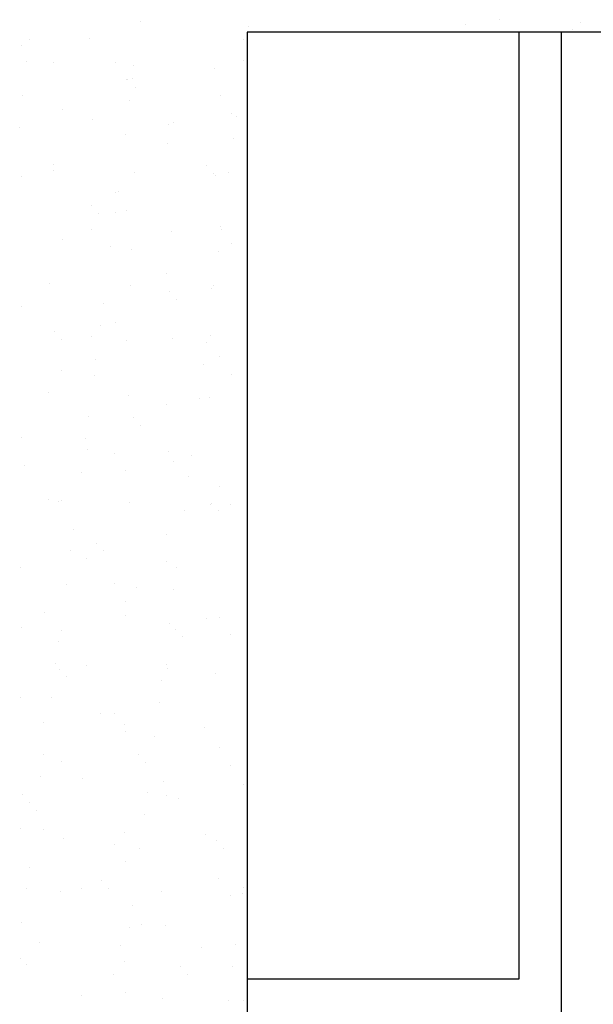
# Model space of a CAD drawing. Units: millimetres. Extents: x -857 to 54106, y -13666 to 13947.
# Tile 36 of 41: x 31477 to 32096, y 9453 to 10516. Entities that reach past the tile are written whole.
import ezdxf

# ---------------------------------------------------------------- set-up
doc = ezdxf.new("R2010")
doc.units = ezdxf.units.MM
for name, color, linetype in [('A-FRN', 11, 'Continuous'), ('A-HT', 15, 'Continuous'), ('L-HT', 1, 'Continuous')]:
    doc.layers.add(name, color=color, linetype=linetype)
doc.layers.add('A-FURN', color=21, linetype='Continuous', lineweight=18)

# ---------------------------------------------------------------- blocks, each defined once
blk = doc.blocks.new('*X18')
at = {"color": 0}
for p, q in [((1.2165, 2.3691), (1.2165, 2.3691)), ((1.2758, 2.3687), (1.2758, 2.3687)), ((1.3141, 2.3717), (1.3141, 2.3717)), ((1.3722, 2.3694), (1.3722, 2.3694)), ((1.5279, 2.3697), (1.5279, 2.3697)), ((1.6837, 2.37), (1.6837, 2.37)), ((1.7172, 2.3656), (1.7172, 2.3656)), ((1.8394, 2.3703), (1.8394, 2.3703)), ((1.911, 2.3696), (1.911, 2.3696)), ((1.9951, 2.3706), (1.9951, 2.3706)), ((2.1111, 2.3679), (2.1111, 2.3679)), ((2.1508, 2.3708), (2.1508, 2.3708)), ((2.264, 2.3694), (2.264, 2.3694)), ((2.3065, 2.3711), (2.3065, 2.3711)), ((1.2091, 2.36), (1.2091, 2.36)), ((1.2351, 2.3634), (1.2351, 2.3634)), ((2.1203, 2.3595), (2.1203, 2.3595)), ((2.1973, 2.3606), (2.1973, 2.3606)), ((2.2234, 2.364), (2.2234, 2.364)), ((2.3141, 2.3635), (2.3141, 2.3635)), ((1.8936, 2.3418), (1.8936, 2.3418)), ((2.0244, 2.3435), (2.0244, 2.3435)), ((2.0627, 2.3429), (2.0627, 2.3429)), ((2.0888, 2.3463), (2.0888, 2.3463)), ((2.1294, 2.3517), (2.1294, 2.3517)), ((2.1523, 2.3429), (2.1523, 2.3429)), ((2.2874, 2.3477), (2.2874, 2.3477)), ((1.2368, 2.3316), (1.2368, 2.3316)), ((1.3576, 2.3319), (1.3576, 2.3319)), ((1.3647, 2.331), (1.3647, 2.331)), ((1.4997, 2.3359), (1.4997, 2.3359)), ((1.5577, 2.3302), (1.5577, 2.3302)), ((1.6306, 2.3375), (1.6306, 2.3375)), ((1.7585, 2.3369), (1.7585, 2.3369)), ((1.9948, 2.3339), (1.9948, 2.3339)), ((1.2924, 2.3208), (1.2924, 2.3208)), ((1.4481, 2.3211), (1.4481, 2.3211)), ((1.5669, 2.3217), (1.5669, 2.3217)), ((1.6038, 2.3214), (1.6038, 2.3214)), ((1.7596, 2.3216), (1.7596, 2.3216)), ((1.7607, 2.3257), (1.7607, 2.3257)), ((1.9153, 2.3219), (1.9153, 2.3219)), ((1.9282, 2.3252), (1.9282, 2.3252)), ((1.9542, 2.3286), (1.9542, 2.3286)), ((1.9608, 2.324), (1.9608, 2.324)), ((2.071, 2.3222), (2.071, 2.3222)), ((2.1638, 2.3196), (2.1638, 2.3196)), ((2.2267, 2.3225), (2.2267, 2.3225)), ((1.7936, 2.3074), (1.7936, 2.3074)), ((1.8196, 2.3109), (1.8196, 2.3109)), ((1.8602, 2.3162), (1.8602, 2.3162)), ((1.97, 2.3156), (1.97, 2.3156)), ((1.7256, 2.2985), (1.7256, 2.2985)), ((2.092, 2.2966), (2.092, 2.2966)), ((2.2229, 2.2983), (2.2229, 2.2983)), ((2.3508, 2.2976), (2.3508, 2.2976)), ((1.2073, 2.288), (1.2073, 2.288)), ((1.3044, 2.2847), (1.3044, 2.2847)), ((1.4074, 2.2863), (1.4074, 2.2863)), ((1.4353, 2.2864), (1.4353, 2.2864)), ((1.5632, 2.2858), (1.5632, 2.2858)), ((1.6104, 2.2819), (1.6104, 2.2819)), ((1.659, 2.2897), (1.659, 2.2897)), ((1.685, 2.2932), (1.685, 2.2932)), ((1.6982, 2.2907), (1.6982, 2.2907)), ((1.8291, 2.2923), (1.8291, 2.2923)), ((1.957, 2.2917), (1.957, 2.2917)), ((1.4166, 2.2778), (1.4166, 2.2778)), ((1.5244, 2.272), (1.5244, 2.272)), ((1.5504, 2.2754), (1.5504, 2.2754)), ((1.5911, 2.2808), (1.5911, 2.2808)), ((1.8105, 2.2801), (1.8105, 2.2801)), ((1.8197, 2.2717), (1.8197, 2.2717)), ((2.0135, 2.2757), (2.0135, 2.2757)), ((2.2136, 2.274), (2.2136, 2.274)), ((1.4565, 2.2631), (1.4565, 2.2631)), ((1.8587, 2.2585), (1.8587, 2.2585)), ((2.0144, 2.2588), (2.0144, 2.2588)), ((2.1701, 2.2591), (2.1701, 2.2591)), ((2.2228, 2.2656), (2.2228, 2.2656)), ((2.3258, 2.2594), (2.3258, 2.2594)), ((1.2358, 2.2574), (1.2358, 2.2574)), ((1.3898, 2.2543), (1.3898, 2.2543)), ((1.3915, 2.2577), (1.3915, 2.2577)), ((1.4158, 2.2577), (1.4158, 2.2577)), ((1.5472, 2.2579), (1.5472, 2.2579)), ((1.7029, 2.2582), (1.7029, 2.2582)), ((2.0276, 2.2471), (2.0276, 2.2471)), ((2.2905, 2.2514), (2.2905, 2.2514)), ((1.2399, 2.2353), (1.2399, 2.2353)), ((1.2552, 2.2366), (1.2552, 2.2366)), ((1.2569, 2.2439), (1.2569, 2.2439)), ((1.2571, 2.2424), (1.2571, 2.2424)), ((1.2812, 2.24), (1.2812, 2.24)), ((1.3219, 2.2453), (1.3219, 2.2453)), ((1.4126, 2.2442), (1.4126, 2.2442)), ((1.4601, 2.238), (1.4601, 2.238)), ((1.5029, 2.2395), (1.5029, 2.2395)), ((1.5683, 2.2445), (1.5683, 2.2445)), ((1.6338, 2.2412), (1.6338, 2.2412)), ((1.6602, 2.2363), (1.6602, 2.2363)), ((1.724, 2.2448), (1.724, 2.2448)), ((1.7617, 2.2406), (1.7617, 2.2406)), ((1.8797, 2.2451), (1.8797, 2.2451)), ((1.8967, 2.2455), (1.8967, 2.2455)), ((2.0354, 2.2454), (2.0354, 2.2454)), ((2.1555, 2.2465), (2.1555, 2.2465)), ((2.1912, 2.2456), (2.1912, 2.2456)), ((2.2434, 2.2372), (2.2434, 2.2372)), ((2.2695, 2.2406), (2.2695, 2.2406)), ((2.3101, 2.246), (2.3101, 2.246)), ((2.3469, 2.2459), (2.3469, 2.2459)), ((1.1873, 2.2276), (1.1873, 2.2276)), ((1.2663, 2.234), (1.2663, 2.234)), ((1.3678, 2.2347), (1.3678, 2.2347)), ((1.6694, 2.2278), (1.6694, 2.2278)), ((1.8632, 2.2318), (1.8632, 2.2318)), ((2.0633, 2.2301), (2.0633, 2.2301)), ((2.1755, 2.2283), (2.1755, 2.2283)), ((2.2663, 2.2257), (2.2663, 2.2257)), ((2.0725, 2.2217), (2.0725, 2.2217)), ((2.1088, 2.2195), (2.1088, 2.2195)), ((2.1349, 2.2229), (2.1349, 2.2229)), ((1.9743, 2.2018), (1.9743, 2.2018)), ((2.0003, 2.2052), (2.0003, 2.2052)), ((2.0409, 2.2106), (2.0409, 2.2106)), ((2.0952, 2.2002), (2.0952, 2.2002)), ((2.2261, 2.2019), (2.2261, 2.2019)), ((2.354, 2.2013), (2.354, 2.2013)), ((1.3075, 2.1884), (1.3075, 2.1884)), ((1.3098, 2.1941), (1.3098, 2.1941)), ((1.3328, 2.1956), (1.3328, 2.1956)), ((1.4384, 2.1901), (1.4384, 2.1901)), ((1.4885, 2.1959), (1.4885, 2.1959)), ((1.5099, 2.1924), (1.5099, 2.1924)), ((1.5663, 2.1895), (1.5663, 2.1895)), ((1.6442, 2.1961), (1.6442, 2.1961)), ((1.7014, 2.1943), (1.7014, 2.1943)), ((1.7129, 2.188), (1.7129, 2.188)), ((1.7999, 2.1964), (1.7999, 2.1964)), ((1.8322, 2.196), (1.8322, 2.196)), ((1.9063, 2.1928), (1.9063, 2.1928)), ((1.9556, 2.1967), (1.9556, 2.1967)), ((1.9601, 2.1954), (1.9601, 2.1954)), ((2.1114, 2.197), (2.1114, 2.197)), ((2.2671, 2.1973), (2.2671, 2.1973)), ((1.5191, 2.1839), (1.5191, 2.1839)), ((1.8397, 2.1841), (1.8397, 2.1841)), ((1.8657, 2.1875), (1.8657, 2.1875)), ((1.913, 2.1862), (1.913, 2.1862)), ((1.9222, 2.1778), (1.9222, 2.1778)), ((2.116, 2.1818), (2.116, 2.1818)), ((2.3161, 2.1801), (2.3161, 2.1801)), ((1.7051, 2.1663), (1.7051, 2.1663)), ((1.7311, 2.1698), (1.7311, 2.1698)), ((1.7717, 2.1751), (1.7717, 2.1751)), ((2.3253, 2.1717), (2.3253, 2.1717)), ((1.6372, 2.1574), (1.6372, 2.1574)), ((2.2937, 2.155), (2.2937, 2.155)), ((1.3596, 2.1485), (1.3596, 2.1485)), ((1.506, 2.1432), (1.506, 2.1432)), ((1.5626, 2.1441), (1.5626, 2.1441)), ((1.5705, 2.1486), (1.5705, 2.1486)), ((1.5965, 2.152), (1.5965, 2.152)), ((1.6369, 2.1449), (1.6369, 2.1449)), ((1.7627, 2.1424), (1.7627, 2.1424)), ((1.7648, 2.1442), (1.7648, 2.1442)), ((1.8999, 2.1491), (1.8999, 2.1491)), ((2.0307, 2.1508), (2.0307, 2.1508)), ((2.1586, 2.1502), (2.1586, 2.1502)), ((1.2431, 2.1389), (1.2431, 2.1389)), ((1.2762, 2.1322), (1.2762, 2.1322)), ((1.3688, 2.14), (1.3688, 2.14)), ((1.371, 2.1383), (1.371, 2.1383)), ((1.4319, 2.1324), (1.4319, 2.1324)), ((1.4359, 2.1309), (1.4359, 2.1309)), ((1.4619, 2.1343), (1.4619, 2.1343)), ((1.5026, 2.1397), (1.5026, 2.1397)), ((1.5876, 2.1327), (1.5876, 2.1327)), ((1.7433, 2.133), (1.7433, 2.133)), ((1.7719, 2.1339), (1.7719, 2.1339)), ((1.899, 2.1333), (1.899, 2.1333)), ((1.9657, 2.1379), (1.9657, 2.1379)), ((2.0547, 2.1336), (2.0547, 2.1336)), ((2.1658, 2.1362), (2.1658, 2.1362)), ((2.2105, 2.1339), (2.2105, 2.1339)), ((1.2973, 2.1187), (1.2973, 2.1187)), ((1.368, 2.122), (1.368, 2.122)), ((1.453, 2.119), (1.453, 2.119)), ((1.6087, 2.1193), (1.6087, 2.1193)), ((1.7644, 2.1196), (1.7644, 2.1196)), ((1.9201, 2.1199), (1.9201, 2.1199)), ((2.0758, 2.1201), (2.0758, 2.1201)), ((2.175, 2.1278), (2.175, 2.1278)), ((2.2315, 2.1204), (2.2315, 2.1204)), ((2.3156, 2.1173), (2.3156, 2.1173)), ((2.3562, 2.1226), (2.3562, 2.1226)), ((1.3013, 2.1132), (1.3013, 2.1132)), ((1.3273, 2.1166), (1.3273, 2.1166)), ((2.2292, 2.1056), (2.2292, 2.1056)), ((2.2895, 2.1138), (2.2895, 2.1138)), ((1.1927, 2.0989), (1.1927, 2.0989)), ((1.2093, 2.1046), (1.2093, 2.1046)), ((1.2334, 2.1042), (1.2334, 2.1042)), ((1.4123, 2.1002), (1.4123, 2.1002)), ((2.0983, 2.1039), (2.0983, 2.1039)), ((2.2216, 2.1049), (2.2216, 2.1049)), ((2.3571, 2.105), (2.3571, 2.105)), ((1.191, 1.8397), (1.191, 1.8397)), ((1.1851, 1.7982), (1.1851, 1.7982)), ((1.1965, 1.711), (1.1965, 1.711)), ((1.1882, 1.7018), (1.1882, 1.7018))]:
    blk.add_line(p, q, dxfattribs=at)
blk = doc.blocks.new('A$C6796526C')
at = {"layer": 'A-FRN'}
blk.add_lwpolyline([(0.65, 2.8), (0.65, 0.9), (2.25, 0.9), (2.25, 2.8)], dxfattribs=at)
at = {"layer": 'L-HT'}
for p, q in [((0.65, 1.2749), (2.25, 1.2749)), ((1.7809, 1.2249), (0.65, 1.2249)), ((1.7809, 0.9), (1.7809, 1.2249))]:
    blk.add_line(p, q, dxfattribs=at)
at = {"layer": 'A-HT', "extrusion": (0, 0, -1), "zscale": -1, "rotation": 180}
blk.add_blockref('*X18', (0.55, 3), dxfattribs=at)

msp = doc.modelspace()

# ---------------------------------------------------------------- block references
at = {"layer": 'A-FURN', "xscale": 903.6084929786902, "yscale": 903.6084929786902, "zscale": 903.6084929786902, "rotation": 269.9999999999988}
msp.add_blockref('A$C6796526C', (30909.253, 11089.463), dxfattribs=at)

doc.saveas('drawing.dxf')
